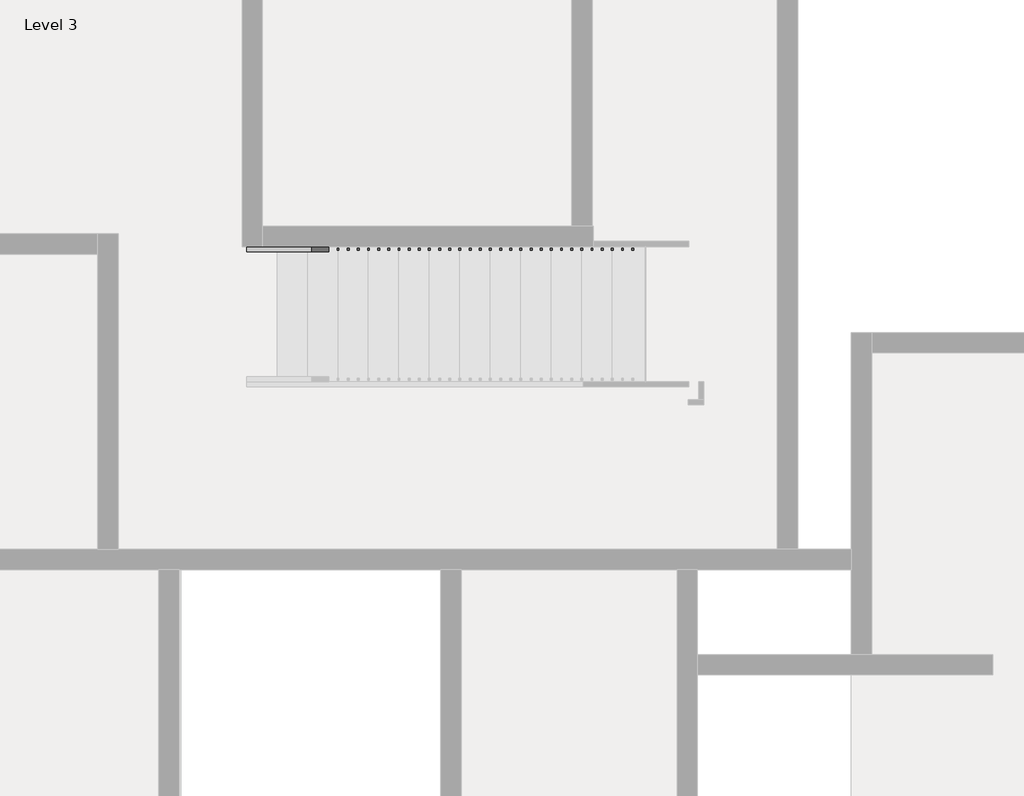
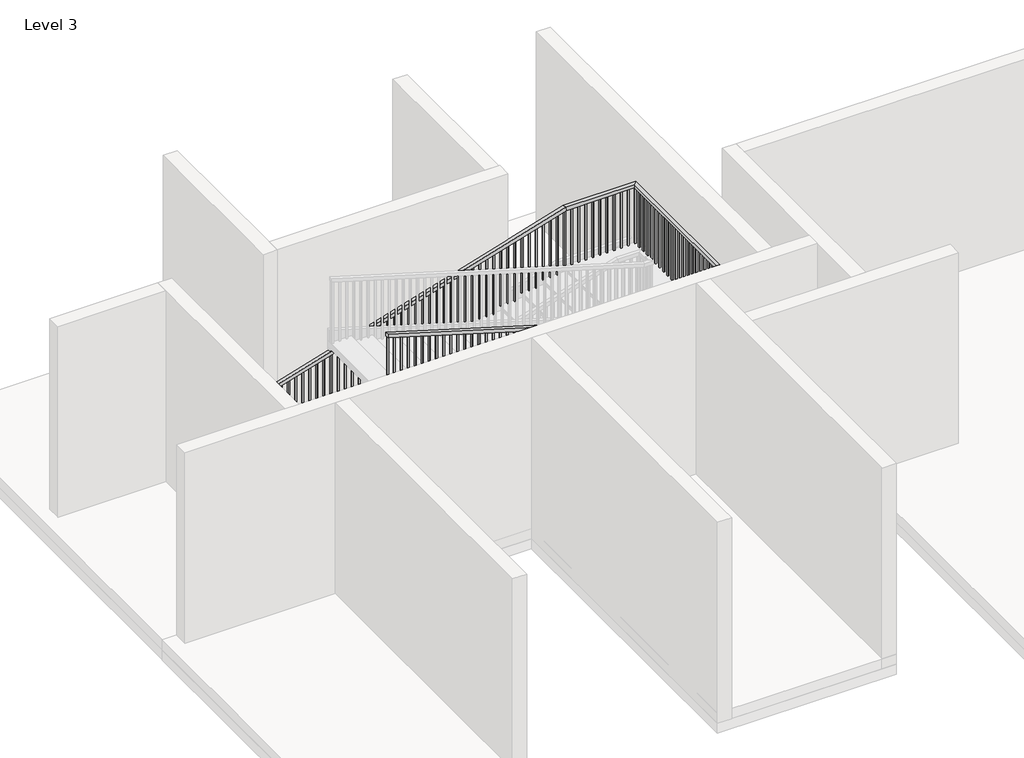
# One storey, part 10 of 14: 1 railing.
"""IFC4 building model written with IfcOpenShell, lengths in millimetres."""

from ifc_helpers import new_model, si_unit, frame, origin, place, context, project, spatial, polyline, outline, extrude, faceted_brep, element, save

model = new_model("IFC4")

# Units and contexts
model_context = context("Model", 3, world=origin())
ifc_project = project(units=[si_unit("LENGTHUNIT", "METRE", prefix="MILLI")], contexts=[model_context])

# Site, building, storey
site = spatial("IfcSite", under=ifc_project)
building = spatial("IfcBuilding", under=site)
storey = spatial("IfcBuildingStorey", under=building, Name="Level 3", Elevation=6096.0)

# Railing
placement = place(None, origin())
element("IfcRailing", 1, ObjectType="Handrail - Rectangular", at=placement, inside=storey, context=model_context, shape_type="SolidModel", body=[
    faceted_brep([(-5254.0891351, 12506.0715905, 7101.84), (-5254.0891351, 12506.0715905, 7048.8032429), (-5254.0891351, 12455.2715905, 7048.8032429), (-5254.0891351, 12455.2715905, 7101.84), (-986.8891351, 12506.0715905, 8382.0), (-979.4332782, 12506.0715905, 8331.2), (-979.4332782, 12455.2715905, 8331.2), (-986.8891351, 12455.2715905, 8382.0), (54.5108649, 12506.0715905, 8382.0), (54.5108649, 12506.0715905, 8331.2), (3.7108649, 12455.2715905, 8331.2), (3.7108649, 12455.2715905, 8382.0), (54.5108649, 9478.4949943, 8382.0), (54.5108649, 9478.4949943, 8331.2), (3.7108649, 9529.2949943, 8331.2), (3.7108649, 9529.2949943, 8382.0), (-682.0891351, 9478.4949943, 8382.0), (-689.544992, 9478.4949943, 8331.2), (-689.544992, 9529.2949943, 8331.2), (-682.0891351, 9529.2949943, 8382.0), (-5254.0891351, 9478.4949943, 9753.6), (-5254.0891351, 9529.2949943, 9753.6), (-5254.0891351, 9529.2949943, 9700.5632429), (-5254.0891351, 9478.4949943, 9700.5632429)], [[[0, 1, 2, 3]], [[1, 0, 4, 5]], [[2, 1, 5, 6]], [[3, 2, 6, 7]], [[0, 3, 7, 4]], [[5, 4, 8, 9]], [[6, 5, 9, 10]], [[7, 6, 10, 11]], [[4, 7, 11, 8]], [[9, 8, 12, 13]], [[10, 9, 13, 14]], [[11, 10, 14, 15]], [[8, 11, 15, 12]], [[13, 12, 16, 17]], [[14, 13, 17, 18]], [[15, 14, 18, 19]], [[12, 15, 19, 16]], [[20, 21, 22, 23]], [[17, 16, 20, 23]], [[18, 17, 23, 22]], [[19, 18, 22, 21]], [[16, 19, 21, 20]]]),
    extrude(outline(polyline([(9672.9407429, -5162.0141351), (8747.76, -5162.0141351), (8747.76, -5142.9641351), (9667.2257429, -5142.9641351), (9672.9407429, -5162.0141351)])), frame((0.0, 9494.3699943, 0.0), z_axis=(0.0, 1.0, 0.0), x_axis=(0.0, 0.0, 1.0)), (0.0, 0.0, 1.0), 19.05),
    extrude(outline(polyline([(9642.4607429, -5060.4141351), (8747.76, -5060.4141351), (8747.76, -5041.3641351), (9636.7457429, -5041.3641351), (9642.4607429, -5060.4141351)])), frame((0.0, 9494.3699943, 0.0), z_axis=(0.0, 1.0, 0.0), x_axis=(0.0, 0.0, 1.0)), (0.0, 0.0, 1.0), 19.05),
    extrude(outline(polyline([(9611.9807429, -4958.8141351), (8747.76, -4958.8141351), (8747.76, -4939.7641351), (9606.2657429, -4939.7641351), (9611.9807429, -4958.8141351)])), frame((0.0, 9494.3699943, 0.0), z_axis=(0.0, 1.0, 0.0), x_axis=(0.0, 0.0, 1.0)), (0.0, 0.0, 1.0), 19.05),
    extrude(outline(polyline([(9581.5007429, -4857.2141351), (8656.32, -4857.2141351), (8656.32, -4838.1641351), (9575.7857429, -4838.1641351), (9581.5007429, -4857.2141351)])), frame((0.0, 9494.3699943, 0.0), z_axis=(0.0, 1.0, 0.0), x_axis=(0.0, 0.0, 1.0)), (0.0, 0.0, 1.0), 19.05),
    extrude(outline(polyline([(9551.0207429, -4755.6141351), (8656.32, -4755.6141351), (8656.32, -4736.5641351), (9545.3057429, -4736.5641351), (9551.0207429, -4755.6141351)])), frame((0.0, 9494.3699943, 0.0), z_axis=(0.0, 1.0, 0.0), x_axis=(0.0, 0.0, 1.0)), (0.0, 0.0, 1.0), 19.05),
    extrude(outline(polyline([(9520.5407429, -4654.0141351), (8656.32, -4654.0141351), (8656.32, -4634.9641351), (9514.8257429, -4634.9641351), (9520.5407429, -4654.0141351)])), frame((0.0, 9494.3699943, 0.0), z_axis=(0.0, 1.0, 0.0), x_axis=(0.0, 0.0, 1.0)), (0.0, 0.0, 1.0), 19.05),
    extrude(outline(polyline([(9490.0607429, -4552.4141351), (8564.88, -4552.4141351), (8564.88, -4533.3641351), (9484.3457429, -4533.3641351), (9490.0607429, -4552.4141351)])), frame((0.0, 9494.3699943, 0.0), z_axis=(0.0, 1.0, 0.0), x_axis=(0.0, 0.0, 1.0)), (0.0, 0.0, 1.0), 19.05),
    extrude(outline(polyline([(9459.5807429, -4450.8141351), (8564.88, -4450.8141351), (8564.88, -4431.7641351), (9453.8657429, -4431.7641351), (9459.5807429, -4450.8141351)])), frame((0.0, 9494.3699943, 0.0), z_axis=(0.0, 1.0, 0.0), x_axis=(0.0, 0.0, 1.0)), (0.0, 0.0, 1.0), 19.05),
    extrude(outline(polyline([(9429.1007429, -4349.2141351), (8564.88, -4349.2141351), (8564.88, -4330.1641351), (9423.3857429, -4330.1641351), (9429.1007429, -4349.2141351)])), frame((0.0, 9494.3699943, 0.0), z_axis=(0.0, 1.0, 0.0), x_axis=(0.0, 0.0, 1.0)), (0.0, 0.0, 1.0), 19.05),
    extrude(outline(polyline([(9398.6207429, -4247.6141351), (8473.44, -4247.6141351), (8473.44, -4228.5641351), (9392.9057429, -4228.5641351), (9398.6207429, -4247.6141351)])), frame((0.0, 9494.3699943, 0.0), z_axis=(0.0, 1.0, 0.0), x_axis=(0.0, 0.0, 1.0)), (0.0, 0.0, 1.0), 19.05),
    extrude(outline(polyline([(9368.1407429, -4146.0141351), (8473.44, -4146.0141351), (8473.44, -4126.9641351), (9362.4257429, -4126.9641351), (9368.1407429, -4146.0141351)])), frame((0.0, 9494.3699943, 0.0), z_axis=(0.0, 1.0, 0.0), x_axis=(0.0, 0.0, 1.0)), (0.0, 0.0, 1.0), 19.05),
    extrude(outline(polyline([(9337.6607429, -4044.4141351), (8473.44, -4044.4141351), (8473.44, -4025.3641351), (9331.9457429, -4025.3641351), (9337.6607429, -4044.4141351)])), frame((0.0, 9494.3699943, 0.0), z_axis=(0.0, 1.0, 0.0), x_axis=(0.0, 0.0, 1.0)), (0.0, 0.0, 1.0), 19.05),
    extrude(outline(polyline([(9307.1807429, -3942.8141351), (8382.0, -3942.8141351), (8382.0, -3923.7641351), (9301.4657429, -3923.7641351), (9307.1807429, -3942.8141351)])), frame((0.0, 9494.3699943, 0.0), z_axis=(0.0, 1.0, 0.0), x_axis=(0.0, 0.0, 1.0)), (0.0, 0.0, 1.0), 19.05),
    extrude(outline(polyline([(9276.7007429, -3841.2141351), (8382.0, -3841.2141351), (8382.0, -3822.1641351), (9270.9857429, -3822.1641351), (9276.7007429, -3841.2141351)])), frame((0.0, 9494.3699943, 0.0), z_axis=(0.0, 1.0, 0.0), x_axis=(0.0, 0.0, 1.0)), (0.0, 0.0, 1.0), 19.05),
    extrude(outline(polyline([(9246.2207429, -3739.6141351), (8382.0, -3739.6141351), (8382.0, -3720.5641351), (9240.5057429, -3720.5641351), (9246.2207429, -3739.6141351)])), frame((0.0, 9494.3699943, 0.0), z_axis=(0.0, 1.0, 0.0), x_axis=(0.0, 0.0, 1.0)), (0.0, 0.0, 1.0), 19.05),
    extrude(outline(polyline([(9215.7407429, -3638.0141351), (8290.56, -3638.0141351), (8290.56, -3618.9641351), (9210.0257429, -3618.9641351), (9215.7407429, -3638.0141351)])), frame((0.0, 9494.3699943, 0.0), z_axis=(0.0, 1.0, 0.0), x_axis=(0.0, 0.0, 1.0)), (0.0, 0.0, 1.0), 19.05),
    extrude(outline(polyline([(9185.2607429, -3536.4141351), (8290.56, -3536.4141351), (8290.56, -3517.3641351), (9179.5457429, -3517.3641351), (9185.2607429, -3536.4141351)])), frame((0.0, 9494.3699943, 0.0), z_axis=(0.0, 1.0, 0.0), x_axis=(0.0, 0.0, 1.0)), (0.0, 0.0, 1.0), 19.05),
    extrude(outline(polyline([(9154.7807429, -3434.8141351), (8290.56, -3434.8141351), (8290.56, -3415.7641351), (9149.0657429, -3415.7641351), (9154.7807429, -3434.8141351)])), frame((0.0, 9494.3699943, 0.0), z_axis=(0.0, 1.0, 0.0), x_axis=(0.0, 0.0, 1.0)), (0.0, 0.0, 1.0), 19.05),
    extrude(outline(polyline([(9124.3007429, -3333.2141351), (8199.12, -3333.2141351), (8199.12, -3314.1641351), (9118.5857429, -3314.1641351), (9124.3007429, -3333.2141351)])), frame((0.0, 9494.3699943, 0.0), z_axis=(0.0, 1.0, 0.0), x_axis=(0.0, 0.0, 1.0)), (0.0, 0.0, 1.0), 19.05),
    extrude(outline(polyline([(9093.8207429, -3231.6141351), (8199.12, -3231.6141351), (8199.12, -3212.5641351), (9088.1057429, -3212.5641351), (9093.8207429, -3231.6141351)])), frame((0.0, 9494.3699943, 0.0), z_axis=(0.0, 1.0, 0.0), x_axis=(0.0, 0.0, 1.0)), (0.0, 0.0, 1.0), 19.05),
    extrude(outline(polyline([(9063.3407429, -3130.0141351), (8199.12, -3130.0141351), (8199.12, -3110.9641351), (9057.6257429, -3110.9641351), (9063.3407429, -3130.0141351)])), frame((0.0, 9494.3699943, 0.0), z_axis=(0.0, 1.0, 0.0), x_axis=(0.0, 0.0, 1.0)), (0.0, 0.0, 1.0), 19.05),
    extrude(outline(polyline([(9032.8607429, -3028.4141351), (8107.68, -3028.4141351), (8107.68, -3009.3641351), (9027.1457429, -3009.3641351), (9032.8607429, -3028.4141351)])), frame((0.0, 9494.3699943, 0.0), z_axis=(0.0, 1.0, 0.0), x_axis=(0.0, 0.0, 1.0)), (0.0, 0.0, 1.0), 19.05),
    extrude(outline(polyline([(9002.3807429, -2926.8141351), (8107.68, -2926.8141351), (8107.68, -2907.7641351), (8996.6657429, -2907.7641351), (9002.3807429, -2926.8141351)])), frame((0.0, 9494.3699943, 0.0), z_axis=(0.0, 1.0, 0.0), x_axis=(0.0, 0.0, 1.0)), (0.0, 0.0, 1.0), 19.05),
    extrude(outline(polyline([(8971.9007429, -2825.2141351), (8107.68, -2825.2141351), (8107.68, -2806.1641351), (8966.1857429, -2806.1641351), (8971.9007429, -2825.2141351)])), frame((0.0, 9494.3699943, 0.0), z_axis=(0.0, 1.0, 0.0), x_axis=(0.0, 0.0, 1.0)), (0.0, 0.0, 1.0), 19.05),
    extrude(outline(polyline([(8941.4207429, -2723.6141351), (8016.24, -2723.6141351), (8016.24, -2704.5641351), (8935.7057429, -2704.5641351), (8941.4207429, -2723.6141351)])), frame((0.0, 9494.3699943, 0.0), z_axis=(0.0, 1.0, 0.0), x_axis=(0.0, 0.0, 1.0)), (0.0, 0.0, 1.0), 19.05),
    extrude(outline(polyline([(8910.9407429, -2622.0141351), (8016.24, -2622.0141351), (8016.24, -2602.9641351), (8905.2257429, -2602.9641351), (8910.9407429, -2622.0141351)])), frame((0.0, 9494.3699943, 0.0), z_axis=(0.0, 1.0, 0.0), x_axis=(0.0, 0.0, 1.0)), (0.0, 0.0, 1.0), 19.05),
    extrude(outline(polyline([(8880.4607429, -2520.4141351), (8016.24, -2520.4141351), (8016.24, -2501.3641351), (8874.7457429, -2501.3641351), (8880.4607429, -2520.4141351)])), frame((0.0, 9494.3699943, 0.0), z_axis=(0.0, 1.0, 0.0), x_axis=(0.0, 0.0, 1.0)), (0.0, 0.0, 1.0), 19.05),
    extrude(outline(polyline([(8849.9807429, -2418.8141351), (7924.8, -2418.8141351), (7924.8, -2399.7641351), (8844.2657429, -2399.7641351), (8849.9807429, -2418.8141351)])), frame((0.0, 9494.3699943, 0.0), z_axis=(0.0, 1.0, 0.0), x_axis=(0.0, 0.0, 1.0)), (0.0, 0.0, 1.0), 19.05),
    extrude(outline(polyline([(8819.5007429, -2317.2141351), (7924.8, -2317.2141351), (7924.8, -2298.1641351), (8813.7857429, -2298.1641351), (8819.5007429, -2317.2141351)])), frame((0.0, 9494.3699943, 0.0), z_axis=(0.0, 1.0, 0.0), x_axis=(0.0, 0.0, 1.0)), (0.0, 0.0, 1.0), 19.05),
    extrude(outline(polyline([(8789.0207429, -2215.6141351), (7924.8, -2215.6141351), (7924.8, -2196.5641351), (8783.3057429, -2196.5641351), (8789.0207429, -2215.6141351)])), frame((0.0, 9494.3699943, 0.0), z_axis=(0.0, 1.0, 0.0), x_axis=(0.0, 0.0, 1.0)), (0.0, 0.0, 1.0), 19.05),
    extrude(outline(polyline([(8758.5407429, -2114.0141351), (7833.36, -2114.0141351), (7833.36, -2094.9641351), (8752.8257429, -2094.9641351), (8758.5407429, -2114.0141351)])), frame((0.0, 9494.3699943, 0.0), z_axis=(0.0, 1.0, 0.0), x_axis=(0.0, 0.0, 1.0)), (0.0, 0.0, 1.0), 19.05),
    extrude(outline(polyline([(8728.0607429, -2012.4141351), (7833.36, -2012.4141351), (7833.36, -1993.3641351), (8722.3457429, -1993.3641351), (8728.0607429, -2012.4141351)])), frame((0.0, 9494.3699943, 0.0), z_axis=(0.0, 1.0, 0.0), x_axis=(0.0, 0.0, 1.0)), (0.0, 0.0, 1.0), 19.05),
    extrude(outline(polyline([(8697.5807429, -1910.8141351), (7833.36, -1910.8141351), (7833.36, -1891.7641351), (8691.8657429, -1891.7641351), (8697.5807429, -1910.8141351)])), frame((0.0, 9494.3699943, 0.0), z_axis=(0.0, 1.0, 0.0), x_axis=(0.0, 0.0, 1.0)), (0.0, 0.0, 1.0), 19.05),
    extrude(outline(polyline([(8667.1007429, -1809.2141351), (7741.92, -1809.2141351), (7741.92, -1790.1641351), (8661.3857429, -1790.1641351), (8667.1007429, -1809.2141351)])), frame((0.0, 9494.3699943, 0.0), z_axis=(0.0, 1.0, 0.0), x_axis=(0.0, 0.0, 1.0)), (0.0, 0.0, 1.0), 19.05),
    extrude(outline(polyline([(8636.6207429, -1707.6141351), (7741.92, -1707.6141351), (7741.92, -1688.5641351), (8630.9057429, -1688.5641351), (8636.6207429, -1707.6141351)])), frame((0.0, 9494.3699943, 0.0), z_axis=(0.0, 1.0, 0.0), x_axis=(0.0, 0.0, 1.0)), (0.0, 0.0, 1.0), 19.05),
    extrude(outline(polyline([(8606.1407429, -1606.0141351), (7741.92, -1606.0141351), (7741.92, -1586.9641351), (8600.4257429, -1586.9641351), (8606.1407429, -1606.0141351)])), frame((0.0, 9494.3699943, 0.0), z_axis=(0.0, 1.0, 0.0), x_axis=(0.0, 0.0, 1.0)), (0.0, 0.0, 1.0), 19.05),
    extrude(outline(polyline([(8575.6607429, -1504.4141351), (7650.48, -1504.4141351), (7650.48, -1485.3641351), (8569.9457429, -1485.3641351), (8575.6607429, -1504.4141351)])), frame((0.0, 9494.3699943, 0.0), z_axis=(0.0, 1.0, 0.0), x_axis=(0.0, 0.0, 1.0)), (0.0, 0.0, 1.0), 19.05),
    extrude(outline(polyline([(8545.1807429, -1402.8141351), (7650.48, -1402.8141351), (7650.48, -1383.7641351), (8539.4657429, -1383.7641351), (8545.1807429, -1402.8141351)])), frame((0.0, 9494.3699943, 0.0), z_axis=(0.0, 1.0, 0.0), x_axis=(0.0, 0.0, 1.0)), (0.0, 0.0, 1.0), 19.05),
    extrude(outline(polyline([(8514.7007429, -1301.2141351), (7650.48, -1301.2141351), (7650.48, -1282.1641351), (8508.9857429, -1282.1641351), (8514.7007429, -1301.2141351)])), frame((0.0, 9494.3699943, 0.0), z_axis=(0.0, 1.0, 0.0), x_axis=(0.0, 0.0, 1.0)), (0.0, 0.0, 1.0), 19.05),
    extrude(outline(polyline([(8484.2207429, -1199.6141351), (7559.04, -1199.6141351), (7559.04, -1180.5641351), (8478.5057429, -1180.5641351), (8484.2207429, -1199.6141351)])), frame((0.0, 9494.3699943, 0.0), z_axis=(0.0, 1.0, 0.0), x_axis=(0.0, 0.0, 1.0)), (0.0, 0.0, 1.0), 19.05),
    extrude(outline(polyline([(8453.7407429, -1098.0141351), (7559.04, -1098.0141351), (7559.04, -1078.9641351), (8448.0257429, -1078.9641351), (8453.7407429, -1098.0141351)])), frame((0.0, 9494.3699943, 0.0), z_axis=(0.0, 1.0, 0.0), x_axis=(0.0, 0.0, 1.0)), (0.0, 0.0, 1.0), 19.05),
    extrude(outline(polyline([(8423.2607429, -996.4141351), (7559.04, -996.4141351), (7559.04, -977.3641351), (8417.5457429, -977.3641351), (8423.2607429, -996.4141351)])), frame((0.0, 9494.3699943, 0.0), z_axis=(0.0, 1.0, 0.0), x_axis=(0.0, 0.0, 1.0)), (0.0, 0.0, 1.0), 19.05),
    extrude(outline(polyline([(8392.7807429, -894.8141351), (7467.6, -894.8141351), (7467.6, -875.7641351), (8387.0657429, -875.7641351), (8392.7807429, -894.8141351)])), frame((0.0, 9494.3699943, 0.0), z_axis=(0.0, 1.0, 0.0), x_axis=(0.0, 0.0, 1.0)), (0.0, 0.0, 1.0), 19.05),
    extrude(outline(polyline([(8362.3007429, -793.2141351), (7467.6, -793.2141351), (7467.6, -774.1641351), (8356.5857429, -774.1641351), (8362.3007429, -793.2141351)])), frame((0.0, 9494.3699943, 0.0), z_axis=(0.0, 1.0, 0.0), x_axis=(0.0, 0.0, 1.0)), (0.0, 0.0, 1.0), 19.05),
    extrude(outline(polyline([(-672.5641351, 9494.3699943), (-691.6141351, 9494.3699943), (-691.6141351, 9513.4199943), (-672.5641351, 9513.4199943), (-672.5641351, 9494.3699943)])), frame((0.0, 0.0, 7467.6), z_axis=(0.0, 0.0, 1.0), x_axis=(1.0, 0.0, 0.0)), (0.0, 0.0, 1.0), 863.6),
    extrude(outline(polyline([(-570.9641351, 9494.3699943), (-590.0141351, 9494.3699943), (-590.0141351, 9513.4199943), (-570.9641351, 9513.4199943), (-570.9641351, 9494.3699943)])), frame((0.0, 0.0, 7467.6), z_axis=(0.0, 0.0, 1.0), x_axis=(1.0, 0.0, 0.0)), (0.0, 0.0, 1.0), 863.6),
    extrude(outline(polyline([(-469.3641351, 9494.3699943), (-488.4141351, 9494.3699943), (-488.4141351, 9513.4199943), (-469.3641351, 9513.4199943), (-469.3641351, 9494.3699943)])), frame((0.0, 0.0, 7467.6), z_axis=(0.0, 0.0, 1.0), x_axis=(1.0, 0.0, 0.0)), (0.0, 0.0, 1.0), 863.6),
    extrude(outline(polyline([(-367.7641351, 9494.3699943), (-386.8141351, 9494.3699943), (-386.8141351, 9513.4199943), (-367.7641351, 9513.4199943), (-367.7641351, 9494.3699943)])), frame((0.0, 0.0, 7467.6), z_axis=(0.0, 0.0, 1.0), x_axis=(1.0, 0.0, 0.0)), (0.0, 0.0, 1.0), 863.6),
    extrude(outline(polyline([(-266.1641351, 9494.3699943), (-285.2141351, 9494.3699943), (-285.2141351, 9513.4199943), (-266.1641351, 9513.4199943), (-266.1641351, 9494.3699943)])), frame((0.0, 0.0, 7467.6), z_axis=(0.0, 0.0, 1.0), x_axis=(1.0, 0.0, 0.0)), (0.0, 0.0, 1.0), 863.6),
    extrude(outline(polyline([(-164.5641351, 9494.3699943), (-183.6141351, 9494.3699943), (-183.6141351, 9513.4199943), (-164.5641351, 9513.4199943), (-164.5641351, 9494.3699943)])), frame((0.0, 0.0, 7467.6), z_axis=(0.0, 0.0, 1.0), x_axis=(1.0, 0.0, 0.0)), (0.0, 0.0, 1.0), 863.6),
    extrude(outline(polyline([(-62.9641351, 9494.3699943), (-82.0141351, 9494.3699943), (-82.0141351, 9513.4199943), (-62.9641351, 9513.4199943), (-62.9641351, 9494.3699943)])), frame((0.0, 0.0, 7467.6), z_axis=(0.0, 0.0, 1.0), x_axis=(1.0, 0.0, 0.0)), (0.0, 0.0, 1.0), 863.6),
    extrude(outline(polyline([(38.6358649, 9543.7965905), (38.6358649, 9524.7465905), (19.5858649, 9524.7465905), (19.5858649, 9543.7965905), (38.6358649, 9543.7965905)])), frame((0.0, 0.0, 7467.6), z_axis=(0.0, 0.0, 1.0), x_axis=(1.0, 0.0, 0.0)), (0.0, 0.0, 1.0), 863.6),
    extrude(outline(polyline([(38.6358649, 9645.3965905), (38.6358649, 9626.3465905), (19.5858649, 9626.3465905), (19.5858649, 9645.3965905), (38.6358649, 9645.3965905)])), frame((0.0, 0.0, 7467.6), z_axis=(0.0, 0.0, 1.0), x_axis=(1.0, 0.0, 0.0)), (0.0, 0.0, 1.0), 863.6),
    extrude(outline(polyline([(38.6358649, 9746.9965905), (38.6358649, 9727.9465905), (19.5858649, 9727.9465905), (19.5858649, 9746.9965905), (38.6358649, 9746.9965905)])), frame((0.0, 0.0, 7467.6), z_axis=(0.0, 0.0, 1.0), x_axis=(1.0, 0.0, 0.0)), (0.0, 0.0, 1.0), 863.6),
    extrude(outline(polyline([(38.6358649, 9848.5965905), (38.6358649, 9829.5465905), (19.5858649, 9829.5465905), (19.5858649, 9848.5965905), (38.6358649, 9848.5965905)])), frame((0.0, 0.0, 7467.6), z_axis=(0.0, 0.0, 1.0), x_axis=(1.0, 0.0, 0.0)), (0.0, 0.0, 1.0), 863.6),
    extrude(outline(polyline([(38.6358649, 9950.1965905), (38.6358649, 9931.1465905), (19.5858649, 9931.1465905), (19.5858649, 9950.1965905), (38.6358649, 9950.1965905)])), frame((0.0, 0.0, 7467.6), z_axis=(0.0, 0.0, 1.0), x_axis=(1.0, 0.0, 0.0)), (0.0, 0.0, 1.0), 863.6),
    extrude(outline(polyline([(38.6358649, 10051.7965905), (38.6358649, 10032.7465905), (19.5858649, 10032.7465905), (19.5858649, 10051.7965905), (38.6358649, 10051.7965905)])), frame((0.0, 0.0, 7467.6), z_axis=(0.0, 0.0, 1.0), x_axis=(1.0, 0.0, 0.0)), (0.0, 0.0, 1.0), 863.6),
    extrude(outline(polyline([(38.6358649, 10153.3965905), (38.6358649, 10134.3465905), (19.5858649, 10134.3465905), (19.5858649, 10153.3965905), (38.6358649, 10153.3965905)])), frame((0.0, 0.0, 7467.6), z_axis=(0.0, 0.0, 1.0), x_axis=(1.0, 0.0, 0.0)), (0.0, 0.0, 1.0), 863.6),
    extrude(outline(polyline([(38.6358649, 10254.9965905), (38.6358649, 10235.9465905), (19.5858649, 10235.9465905), (19.5858649, 10254.9965905), (38.6358649, 10254.9965905)])), frame((0.0, 0.0, 7467.6), z_axis=(0.0, 0.0, 1.0), x_axis=(1.0, 0.0, 0.0)), (0.0, 0.0, 1.0), 863.6),
    extrude(outline(polyline([(38.6358649, 10356.5965905), (38.6358649, 10337.5465905), (19.5858649, 10337.5465905), (19.5858649, 10356.5965905), (38.6358649, 10356.5965905)])), frame((0.0, 0.0, 7467.6), z_axis=(0.0, 0.0, 1.0), x_axis=(1.0, 0.0, 0.0)), (0.0, 0.0, 1.0), 863.6),
    extrude(outline(polyline([(38.6358649, 10458.1965905), (38.6358649, 10439.1465905), (19.5858649, 10439.1465905), (19.5858649, 10458.1965905), (38.6358649, 10458.1965905)])), frame((0.0, 0.0, 7467.6), z_axis=(0.0, 0.0, 1.0), x_axis=(1.0, 0.0, 0.0)), (0.0, 0.0, 1.0), 863.6),
    extrude(outline(polyline([(38.6358649, 10559.7965905), (38.6358649, 10540.7465905), (19.5858649, 10540.7465905), (19.5858649, 10559.7965905), (38.6358649, 10559.7965905)])), frame((0.0, 0.0, 7467.6), z_axis=(0.0, 0.0, 1.0), x_axis=(1.0, 0.0, 0.0)), (0.0, 0.0, 1.0), 863.6),
    extrude(outline(polyline([(38.6358649, 10661.3965905), (38.6358649, 10642.3465905), (19.5858649, 10642.3465905), (19.5858649, 10661.3965905), (38.6358649, 10661.3965905)])), frame((0.0, 0.0, 7467.6), z_axis=(0.0, 0.0, 1.0), x_axis=(1.0, 0.0, 0.0)), (0.0, 0.0, 1.0), 863.6),
    extrude(outline(polyline([(38.6358649, 10762.9965905), (38.6358649, 10743.9465905), (19.5858649, 10743.9465905), (19.5858649, 10762.9965905), (38.6358649, 10762.9965905)])), frame((0.0, 0.0, 7467.6), z_axis=(0.0, 0.0, 1.0), x_axis=(1.0, 0.0, 0.0)), (0.0, 0.0, 1.0), 863.6),
    extrude(outline(polyline([(38.6358649, 10864.5965905), (38.6358649, 10845.5465905), (19.5858649, 10845.5465905), (19.5858649, 10864.5965905), (38.6358649, 10864.5965905)])), frame((0.0, 0.0, 7467.6), z_axis=(0.0, 0.0, 1.0), x_axis=(1.0, 0.0, 0.0)), (0.0, 0.0, 1.0), 863.6),
    extrude(outline(polyline([(38.6358649, 10966.1965905), (38.6358649, 10947.1465905), (19.5858649, 10947.1465905), (19.5858649, 10966.1965905), (38.6358649, 10966.1965905)])), frame((0.0, 0.0, 7467.6), z_axis=(0.0, 0.0, 1.0), x_axis=(1.0, 0.0, 0.0)), (0.0, 0.0, 1.0), 863.6),
    extrude(outline(polyline([(38.6358649, 11067.7965905), (38.6358649, 11048.7465905), (19.5858649, 11048.7465905), (19.5858649, 11067.7965905), (38.6358649, 11067.7965905)])), frame((0.0, 0.0, 7467.6), z_axis=(0.0, 0.0, 1.0), x_axis=(1.0, 0.0, 0.0)), (0.0, 0.0, 1.0), 863.6),
    extrude(outline(polyline([(38.6358649, 11169.3965905), (38.6358649, 11150.3465905), (19.5858649, 11150.3465905), (19.5858649, 11169.3965905), (38.6358649, 11169.3965905)])), frame((0.0, 0.0, 7467.6), z_axis=(0.0, 0.0, 1.0), x_axis=(1.0, 0.0, 0.0)), (0.0, 0.0, 1.0), 863.6),
    extrude(outline(polyline([(38.6358649, 11270.9965905), (38.6358649, 11251.9465905), (19.5858649, 11251.9465905), (19.5858649, 11270.9965905), (38.6358649, 11270.9965905)])), frame((0.0, 0.0, 7467.6), z_axis=(0.0, 0.0, 1.0), x_axis=(1.0, 0.0, 0.0)), (0.0, 0.0, 1.0), 863.6),
    extrude(outline(polyline([(38.6358649, 11372.5965905), (38.6358649, 11353.5465905), (19.5858649, 11353.5465905), (19.5858649, 11372.5965905), (38.6358649, 11372.5965905)])), frame((0.0, 0.0, 7467.6), z_axis=(0.0, 0.0, 1.0), x_axis=(1.0, 0.0, 0.0)), (0.0, 0.0, 1.0), 863.6),
    extrude(outline(polyline([(38.6358649, 11474.1965905), (38.6358649, 11455.1465905), (19.5858649, 11455.1465905), (19.5858649, 11474.1965905), (38.6358649, 11474.1965905)])), frame((0.0, 0.0, 7467.6), z_axis=(0.0, 0.0, 1.0), x_axis=(1.0, 0.0, 0.0)), (0.0, 0.0, 1.0), 863.6),
    extrude(outline(polyline([(38.6358649, 11575.7965905), (38.6358649, 11556.7465905), (19.5858649, 11556.7465905), (19.5858649, 11575.7965905), (38.6358649, 11575.7965905)])), frame((0.0, 0.0, 7467.6), z_axis=(0.0, 0.0, 1.0), x_axis=(1.0, 0.0, 0.0)), (0.0, 0.0, 1.0), 863.6),
    extrude(outline(polyline([(38.6358649, 11677.3965905), (38.6358649, 11658.3465905), (19.5858649, 11658.3465905), (19.5858649, 11677.3965905), (38.6358649, 11677.3965905)])), frame((0.0, 0.0, 7467.6), z_axis=(0.0, 0.0, 1.0), x_axis=(1.0, 0.0, 0.0)), (0.0, 0.0, 1.0), 863.6),
    extrude(outline(polyline([(38.6358649, 11778.9965905), (38.6358649, 11759.9465905), (19.5858649, 11759.9465905), (19.5858649, 11778.9965905), (38.6358649, 11778.9965905)])), frame((0.0, 0.0, 7467.6), z_axis=(0.0, 0.0, 1.0), x_axis=(1.0, 0.0, 0.0)), (0.0, 0.0, 1.0), 863.6),
    extrude(outline(polyline([(38.6358649, 11880.5965905), (38.6358649, 11861.5465905), (19.5858649, 11861.5465905), (19.5858649, 11880.5965905), (38.6358649, 11880.5965905)])), frame((0.0, 0.0, 7467.6), z_axis=(0.0, 0.0, 1.0), x_axis=(1.0, 0.0, 0.0)), (0.0, 0.0, 1.0), 863.6),
    extrude(outline(polyline([(38.6358649, 11982.1965905), (38.6358649, 11963.1465905), (19.5858649, 11963.1465905), (19.5858649, 11982.1965905), (38.6358649, 11982.1965905)])), frame((0.0, 0.0, 7467.6), z_axis=(0.0, 0.0, 1.0), x_axis=(1.0, 0.0, 0.0)), (0.0, 0.0, 1.0), 863.6),
    extrude(outline(polyline([(38.6358649, 12083.7965905), (38.6358649, 12064.7465905), (19.5858649, 12064.7465905), (19.5858649, 12083.7965905), (38.6358649, 12083.7965905)])), frame((0.0, 0.0, 7467.6), z_axis=(0.0, 0.0, 1.0), x_axis=(1.0, 0.0, 0.0)), (0.0, 0.0, 1.0), 863.6),
    extrude(outline(polyline([(38.6358649, 12185.3965905), (38.6358649, 12166.3465905), (19.5858649, 12166.3465905), (19.5858649, 12185.3965905), (38.6358649, 12185.3965905)])), frame((0.0, 0.0, 7467.6), z_axis=(0.0, 0.0, 1.0), x_axis=(1.0, 0.0, 0.0)), (0.0, 0.0, 1.0), 863.6),
    extrude(outline(polyline([(38.6358649, 12286.9965905), (38.6358649, 12267.9465905), (19.5858649, 12267.9465905), (19.5858649, 12286.9965905), (38.6358649, 12286.9965905)])), frame((0.0, 0.0, 7467.6), z_axis=(0.0, 0.0, 1.0), x_axis=(1.0, 0.0, 0.0)), (0.0, 0.0, 1.0), 863.6),
    extrude(outline(polyline([(38.6358649, 12388.5965905), (38.6358649, 12369.5465905), (19.5858649, 12369.5465905), (19.5858649, 12388.5965905), (38.6358649, 12388.5965905)])), frame((0.0, 0.0, 7467.6), z_axis=(0.0, 0.0, 1.0), x_axis=(1.0, 0.0, 0.0)), (0.0, 0.0, 1.0), 863.6),
    extrude(outline(polyline([(-82.0141351, 12490.1965905), (-62.9641351, 12490.1965905), (-62.9641351, 12471.1465905), (-82.0141351, 12471.1465905), (-82.0141351, 12490.1965905)])), frame((0.0, 0.0, 7467.6), z_axis=(0.0, 0.0, 1.0), x_axis=(1.0, 0.0, 0.0)), (0.0, 0.0, 1.0), 863.6),
    extrude(outline(polyline([(-183.6141351, 12490.1965905), (-164.5641351, 12490.1965905), (-164.5641351, 12471.1465905), (-183.6141351, 12471.1465905), (-183.6141351, 12490.1965905)])), frame((0.0, 0.0, 7467.6), z_axis=(0.0, 0.0, 1.0), x_axis=(1.0, 0.0, 0.0)), (0.0, 0.0, 1.0), 863.6),
    extrude(outline(polyline([(-285.2141351, 12490.1965905), (-266.1641351, 12490.1965905), (-266.1641351, 12471.1465905), (-285.2141351, 12471.1465905), (-285.2141351, 12490.1965905)])), frame((0.0, 0.0, 7467.6), z_axis=(0.0, 0.0, 1.0), x_axis=(1.0, 0.0, 0.0)), (0.0, 0.0, 1.0), 863.6),
    extrude(outline(polyline([(-386.8141351, 12490.1965905), (-367.7641351, 12490.1965905), (-367.7641351, 12471.1465905), (-386.8141351, 12471.1465905), (-386.8141351, 12490.1965905)])), frame((0.0, 0.0, 7467.6), z_axis=(0.0, 0.0, 1.0), x_axis=(1.0, 0.0, 0.0)), (0.0, 0.0, 1.0), 863.6),
    extrude(outline(polyline([(-488.4141351, 12490.1965905), (-469.3641351, 12490.1965905), (-469.3641351, 12471.1465905), (-488.4141351, 12471.1465905), (-488.4141351, 12490.1965905)])), frame((0.0, 0.0, 7467.6), z_axis=(0.0, 0.0, 1.0), x_axis=(1.0, 0.0, 0.0)), (0.0, 0.0, 1.0), 863.6),
    extrude(outline(polyline([(-590.0141351, 12490.1965905), (-570.9641351, 12490.1965905), (-570.9641351, 12471.1465905), (-590.0141351, 12471.1465905), (-590.0141351, 12490.1965905)])), frame((0.0, 0.0, 7467.6), z_axis=(0.0, 0.0, 1.0), x_axis=(1.0, 0.0, 0.0)), (0.0, 0.0, 1.0), 863.6),
    extrude(outline(polyline([(-691.6141351, 12490.1965905), (-672.5641351, 12490.1965905), (-672.5641351, 12471.1465905), (-691.6141351, 12471.1465905), (-691.6141351, 12490.1965905)])), frame((0.0, 0.0, 7467.6), z_axis=(0.0, 0.0, 1.0), x_axis=(1.0, 0.0, 0.0)), (0.0, 0.0, 1.0), 863.6),
    extrude(outline(polyline([(-793.2141351, 12490.1965905), (-774.1641351, 12490.1965905), (-774.1641351, 12471.1465905), (-793.2141351, 12471.1465905), (-793.2141351, 12490.1965905)])), frame((0.0, 0.0, 7467.6), z_axis=(0.0, 0.0, 1.0), x_axis=(1.0, 0.0, 0.0)), (0.0, 0.0, 1.0), 863.6),
    extrude(outline(polyline([(-894.8141351, 12490.1965905), (-875.7641351, 12490.1965905), (-875.7641351, 12471.1465905), (-894.8141351, 12471.1465905), (-894.8141351, 12490.1965905)])), frame((0.0, 0.0, 7467.6), z_axis=(0.0, 0.0, 1.0), x_axis=(1.0, 0.0, 0.0)), (0.0, 0.0, 1.0), 863.6),
    extrude(outline(polyline([(8326.1057429, -996.4141351), (7467.6, -996.4141351), (7467.6, -977.3641351), (8331.8207429, -977.3641351), (8326.1057429, -996.4141351)])), frame((0.0, 12471.1465905, 0.0), z_axis=(0.0, 1.0, 0.0), x_axis=(0.0, 0.0, 1.0)), (0.0, 0.0, 1.0), 19.05),
    extrude(outline(polyline([(8295.6257429, -1098.0141351), (7376.16, -1098.0141351), (7376.16, -1078.9641351), (8301.3407429, -1078.9641351), (8295.6257429, -1098.0141351)])), frame((0.0, 12471.1465905, 0.0), z_axis=(0.0, 1.0, 0.0), x_axis=(0.0, 0.0, 1.0)), (0.0, 0.0, 1.0), 19.05),
    extrude(outline(polyline([(8265.1457429, -1199.6141351), (7376.16, -1199.6141351), (7376.16, -1180.5641351), (8270.8607429, -1180.5641351), (8265.1457429, -1199.6141351)])), frame((0.0, 12471.1465905, 0.0), z_axis=(0.0, 1.0, 0.0), x_axis=(0.0, 0.0, 1.0)), (0.0, 0.0, 1.0), 19.05),
    extrude(outline(polyline([(8234.6657429, -1301.2141351), (7376.16, -1301.2141351), (7376.16, -1282.1641351), (8240.3807429, -1282.1641351), (8234.6657429, -1301.2141351)])), frame((0.0, 12471.1465905, 0.0), z_axis=(0.0, 1.0, 0.0), x_axis=(0.0, 0.0, 1.0)), (0.0, 0.0, 1.0), 19.05),
    extrude(outline(polyline([(8204.1857429, -1402.8141351), (7284.72, -1402.8141351), (7284.72, -1383.7641351), (8209.9007429, -1383.7641351), (8204.1857429, -1402.8141351)])), frame((0.0, 12471.1465905, 0.0), z_axis=(0.0, 1.0, 0.0), x_axis=(0.0, 0.0, 1.0)), (0.0, 0.0, 1.0), 19.05),
    extrude(outline(polyline([(8173.7057429, -1504.4141351), (7284.72, -1504.4141351), (7284.72, -1485.3641351), (8179.4207429, -1485.3641351), (8173.7057429, -1504.4141351)])), frame((0.0, 12471.1465905, 0.0), z_axis=(0.0, 1.0, 0.0), x_axis=(0.0, 0.0, 1.0)), (0.0, 0.0, 1.0), 19.05),
    extrude(outline(polyline([(8143.2257429, -1606.0141351), (7284.72, -1606.0141351), (7284.72, -1586.9641351), (8148.9407429, -1586.9641351), (8143.2257429, -1606.0141351)])), frame((0.0, 12471.1465905, 0.0), z_axis=(0.0, 1.0, 0.0), x_axis=(0.0, 0.0, 1.0)), (0.0, 0.0, 1.0), 19.05),
    extrude(outline(polyline([(8112.7457429, -1707.6141351), (7193.28, -1707.6141351), (7193.28, -1688.5641351), (8118.4607429, -1688.5641351), (8112.7457429, -1707.6141351)])), frame((0.0, 12471.1465905, 0.0), z_axis=(0.0, 1.0, 0.0), x_axis=(0.0, 0.0, 1.0)), (0.0, 0.0, 1.0), 19.05),
    extrude(outline(polyline([(8082.2657429, -1809.2141351), (7193.28, -1809.2141351), (7193.28, -1790.1641351), (8087.9807429, -1790.1641351), (8082.2657429, -1809.2141351)])), frame((0.0, 12471.1465905, 0.0), z_axis=(0.0, 1.0, 0.0), x_axis=(0.0, 0.0, 1.0)), (0.0, 0.0, 1.0), 19.05),
    extrude(outline(polyline([(8051.7857429, -1910.8141351), (7193.28, -1910.8141351), (7193.28, -1891.7641351), (8057.5007429, -1891.7641351), (8051.7857429, -1910.8141351)])), frame((0.0, 12471.1465905, 0.0), z_axis=(0.0, 1.0, 0.0), x_axis=(0.0, 0.0, 1.0)), (0.0, 0.0, 1.0), 19.05),
    extrude(outline(polyline([(8021.3057429, -2012.4141351), (7101.84, -2012.4141351), (7101.84, -1993.3641351), (8027.0207429, -1993.3641351), (8021.3057429, -2012.4141351)])), frame((0.0, 12471.1465905, 0.0), z_axis=(0.0, 1.0, 0.0), x_axis=(0.0, 0.0, 1.0)), (0.0, 0.0, 1.0), 19.05),
    extrude(outline(polyline([(7990.8257429, -2114.0141351), (7101.84, -2114.0141351), (7101.84, -2094.9641351), (7996.5407429, -2094.9641351), (7990.8257429, -2114.0141351)])), frame((0.0, 12471.1465905, 0.0), z_axis=(0.0, 1.0, 0.0), x_axis=(0.0, 0.0, 1.0)), (0.0, 0.0, 1.0), 19.05),
    extrude(outline(polyline([(7960.3457429, -2215.6141351), (7101.84, -2215.6141351), (7101.84, -2196.5641351), (7966.0607429, -2196.5641351), (7960.3457429, -2215.6141351)])), frame((0.0, 12471.1465905, 0.0), z_axis=(0.0, 1.0, 0.0), x_axis=(0.0, 0.0, 1.0)), (0.0, 0.0, 1.0), 19.05),
    extrude(outline(polyline([(7929.8657429, -2317.2141351), (7010.4, -2317.2141351), (7010.4, -2298.1641351), (7935.5807429, -2298.1641351), (7929.8657429, -2317.2141351)])), frame((0.0, 12471.1465905, 0.0), z_axis=(0.0, 1.0, 0.0), x_axis=(0.0, 0.0, 1.0)), (0.0, 0.0, 1.0), 19.05),
    extrude(outline(polyline([(7899.3857429, -2418.8141351), (7010.4, -2418.8141351), (7010.4, -2399.7641351), (7905.1007429, -2399.7641351), (7899.3857429, -2418.8141351)])), frame((0.0, 12471.1465905, 0.0), z_axis=(0.0, 1.0, 0.0), x_axis=(0.0, 0.0, 1.0)), (0.0, 0.0, 1.0), 19.05),
    extrude(outline(polyline([(7868.9057429, -2520.4141351), (7010.4, -2520.4141351), (7010.4, -2501.3641351), (7874.6207429, -2501.3641351), (7868.9057429, -2520.4141351)])), frame((0.0, 12471.1465905, 0.0), z_axis=(0.0, 1.0, 0.0), x_axis=(0.0, 0.0, 1.0)), (0.0, 0.0, 1.0), 19.05),
    extrude(outline(polyline([(7838.4257429, -2622.0141351), (6918.96, -2622.0141351), (6918.96, -2602.9641351), (7844.1407429, -2602.9641351), (7838.4257429, -2622.0141351)])), frame((0.0, 12471.1465905, 0.0), z_axis=(0.0, 1.0, 0.0), x_axis=(0.0, 0.0, 1.0)), (0.0, 0.0, 1.0), 19.05),
    extrude(outline(polyline([(7807.9457429, -2723.6141351), (6918.96, -2723.6141351), (6918.96, -2704.5641351), (7813.6607429, -2704.5641351), (7807.9457429, -2723.6141351)])), frame((0.0, 12471.1465905, 0.0), z_axis=(0.0, 1.0, 0.0), x_axis=(0.0, 0.0, 1.0)), (0.0, 0.0, 1.0), 19.05),
    extrude(outline(polyline([(7777.4657429, -2825.2141351), (6918.96, -2825.2141351), (6918.96, -2806.1641351), (7783.1807429, -2806.1641351), (7777.4657429, -2825.2141351)])), frame((0.0, 12471.1465905, 0.0), z_axis=(0.0, 1.0, 0.0), x_axis=(0.0, 0.0, 1.0)), (0.0, 0.0, 1.0), 19.05),
    extrude(outline(polyline([(7746.9857429, -2926.8141351), (6827.52, -2926.8141351), (6827.52, -2907.7641351), (7752.7007429, -2907.7641351), (7746.9857429, -2926.8141351)])), frame((0.0, 12471.1465905, 0.0), z_axis=(0.0, 1.0, 0.0), x_axis=(0.0, 0.0, 1.0)), (0.0, 0.0, 1.0), 19.05),
    extrude(outline(polyline([(7716.5057429, -3028.4141351), (6827.52, -3028.4141351), (6827.52, -3009.3641351), (7722.2207429, -3009.3641351), (7716.5057429, -3028.4141351)])), frame((0.0, 12471.1465905, 0.0), z_axis=(0.0, 1.0, 0.0), x_axis=(0.0, 0.0, 1.0)), (0.0, 0.0, 1.0), 19.05),
    extrude(outline(polyline([(7686.0257429, -3130.0141351), (6827.52, -3130.0141351), (6827.52, -3110.9641351), (7691.7407429, -3110.9641351), (7686.0257429, -3130.0141351)])), frame((0.0, 12471.1465905, 0.0), z_axis=(0.0, 1.0, 0.0), x_axis=(0.0, 0.0, 1.0)), (0.0, 0.0, 1.0), 19.05),
    extrude(outline(polyline([(7655.5457429, -3231.6141351), (6736.08, -3231.6141351), (6736.08, -3212.5641351), (7661.2607429, -3212.5641351), (7655.5457429, -3231.6141351)])), frame((0.0, 12471.1465905, 0.0), z_axis=(0.0, 1.0, 0.0), x_axis=(0.0, 0.0, 1.0)), (0.0, 0.0, 1.0), 19.05),
    extrude(outline(polyline([(7625.0657429, -3333.2141351), (6736.08, -3333.2141351), (6736.08, -3314.1641351), (7630.7807429, -3314.1641351), (7625.0657429, -3333.2141351)])), frame((0.0, 12471.1465905, 0.0), z_axis=(0.0, 1.0, 0.0), x_axis=(0.0, 0.0, 1.0)), (0.0, 0.0, 1.0), 19.05),
    extrude(outline(polyline([(7594.5857429, -3434.8141351), (6736.08, -3434.8141351), (6736.08, -3415.7641351), (7600.3007429, -3415.7641351), (7594.5857429, -3434.8141351)])), frame((0.0, 12471.1465905, 0.0), z_axis=(0.0, 1.0, 0.0), x_axis=(0.0, 0.0, 1.0)), (0.0, 0.0, 1.0), 19.05),
    extrude(outline(polyline([(7564.1057429, -3536.4141351), (6644.64, -3536.4141351), (6644.64, -3517.3641351), (7569.8207429, -3517.3641351), (7564.1057429, -3536.4141351)])), frame((0.0, 12471.1465905, 0.0), z_axis=(0.0, 1.0, 0.0), x_axis=(0.0, 0.0, 1.0)), (0.0, 0.0, 1.0), 19.05),
    extrude(outline(polyline([(7533.6257429, -3638.0141351), (6644.64, -3638.0141351), (6644.64, -3618.9641351), (7539.3407429, -3618.9641351), (7533.6257429, -3638.0141351)])), frame((0.0, 12471.1465905, 0.0), z_axis=(0.0, 1.0, 0.0), x_axis=(0.0, 0.0, 1.0)), (0.0, 0.0, 1.0), 19.05),
    extrude(outline(polyline([(7503.1457429, -3739.6141351), (6644.64, -3739.6141351), (6644.64, -3720.5641351), (7508.8607429, -3720.5641351), (7503.1457429, -3739.6141351)])), frame((0.0, 12471.1465905, 0.0), z_axis=(0.0, 1.0, 0.0), x_axis=(0.0, 0.0, 1.0)), (0.0, 0.0, 1.0), 19.05),
    extrude(outline(polyline([(7472.6657429, -3841.2141351), (6553.2, -3841.2141351), (6553.2, -3822.1641351), (7478.3807429, -3822.1641351), (7472.6657429, -3841.2141351)])), frame((0.0, 12471.1465905, 0.0), z_axis=(0.0, 1.0, 0.0), x_axis=(0.0, 0.0, 1.0)), (0.0, 0.0, 1.0), 19.05),
    extrude(outline(polyline([(7442.1857429, -3942.8141351), (6553.2, -3942.8141351), (6553.2, -3923.7641351), (7447.9007429, -3923.7641351), (7442.1857429, -3942.8141351)])), frame((0.0, 12471.1465905, 0.0), z_axis=(0.0, 1.0, 0.0), x_axis=(0.0, 0.0, 1.0)), (0.0, 0.0, 1.0), 19.05),
    extrude(outline(polyline([(7411.7057429, -4044.4141351), (6553.2, -4044.4141351), (6553.2, -4025.3641351), (7417.4207429, -4025.3641351), (7411.7057429, -4044.4141351)])), frame((0.0, 12471.1465905, 0.0), z_axis=(0.0, 1.0, 0.0), x_axis=(0.0, 0.0, 1.0)), (0.0, 0.0, 1.0), 19.05),
    extrude(outline(polyline([(7381.2257429, -4146.0141351), (6461.76, -4146.0141351), (6461.76, -4126.9641351), (7386.9407429, -4126.9641351), (7381.2257429, -4146.0141351)])), frame((0.0, 12471.1465905, 0.0), z_axis=(0.0, 1.0, 0.0), x_axis=(0.0, 0.0, 1.0)), (0.0, 0.0, 1.0), 19.05),
    extrude(outline(polyline([(7350.7457429, -4247.6141351), (6461.76, -4247.6141351), (6461.76, -4228.5641351), (7356.4607429, -4228.5641351), (7350.7457429, -4247.6141351)])), frame((0.0, 12471.1465905, 0.0), z_axis=(0.0, 1.0, 0.0), x_axis=(0.0, 0.0, 1.0)), (0.0, 0.0, 1.0), 19.05),
    extrude(outline(polyline([(7320.2657429, -4349.2141351), (6461.76, -4349.2141351), (6461.76, -4330.1641351), (7325.9807429, -4330.1641351), (7320.2657429, -4349.2141351)])), frame((0.0, 12471.1465905, 0.0), z_axis=(0.0, 1.0, 0.0), x_axis=(0.0, 0.0, 1.0)), (0.0, 0.0, 1.0), 19.05),
    extrude(outline(polyline([(7289.7857429, -4450.8141351), (6370.32, -4450.8141351), (6370.32, -4431.7641351), (7295.5007429, -4431.7641351), (7289.7857429, -4450.8141351)])), frame((0.0, 12471.1465905, 0.0), z_axis=(0.0, 1.0, 0.0), x_axis=(0.0, 0.0, 1.0)), (0.0, 0.0, 1.0), 19.05),
    extrude(outline(polyline([(7259.3057429, -4552.4141351), (6370.32, -4552.4141351), (6370.32, -4533.3641351), (7265.0207429, -4533.3641351), (7259.3057429, -4552.4141351)])), frame((0.0, 12471.1465905, 0.0), z_axis=(0.0, 1.0, 0.0), x_axis=(0.0, 0.0, 1.0)), (0.0, 0.0, 1.0), 19.05),
    extrude(outline(polyline([(7228.8257429, -4654.0141351), (6370.32, -4654.0141351), (6370.32, -4634.9641351), (7234.5407429, -4634.9641351), (7228.8257429, -4654.0141351)])), frame((0.0, 12471.1465905, 0.0), z_axis=(0.0, 1.0, 0.0), x_axis=(0.0, 0.0, 1.0)), (0.0, 0.0, 1.0), 19.05),
    extrude(outline(polyline([(7198.3457429, -4755.6141351), (6278.88, -4755.6141351), (6278.88, -4736.5641351), (7204.0607429, -4736.5641351), (7198.3457429, -4755.6141351)])), frame((0.0, 12471.1465905, 0.0), z_axis=(0.0, 1.0, 0.0), x_axis=(0.0, 0.0, 1.0)), (0.0, 0.0, 1.0), 19.05),
    extrude(outline(polyline([(7167.8657429, -4857.2141351), (6278.88, -4857.2141351), (6278.88, -4838.1641351), (7173.5807429, -4838.1641351), (7167.8657429, -4857.2141351)])), frame((0.0, 12471.1465905, 0.0), z_axis=(0.0, 1.0, 0.0), x_axis=(0.0, 0.0, 1.0)), (0.0, 0.0, 1.0), 19.05),
    extrude(outline(polyline([(7137.3857429, -4958.8141351), (6278.88, -4958.8141351), (6278.88, -4939.7641351), (7143.1007429, -4939.7641351), (7137.3857429, -4958.8141351)])), frame((0.0, 12471.1465905, 0.0), z_axis=(0.0, 1.0, 0.0), x_axis=(0.0, 0.0, 1.0)), (0.0, 0.0, 1.0), 19.05),
    extrude(outline(polyline([(7106.9057429, -5060.4141351), (6187.44, -5060.4141351), (6187.44, -5041.3641351), (7112.6207429, -5041.3641351), (7106.9057429, -5060.4141351)])), frame((0.0, 12471.1465905, 0.0), z_axis=(0.0, 1.0, 0.0), x_axis=(0.0, 0.0, 1.0)), (0.0, 0.0, 1.0), 19.05),
    extrude(outline(polyline([(7076.4257429, -5162.0141351), (6187.44, -5162.0141351), (6187.44, -5142.9641351), (7082.1407429, -5142.9641351), (7076.4257429, -5162.0141351)])), frame((0.0, 12471.1465905, 0.0), z_axis=(0.0, 1.0, 0.0), x_axis=(0.0, 0.0, 1.0)), (0.0, 0.0, 1.0), 19.05),
    extrude(outline(polyline([(38.6358649, 9513.4199943), (38.6358649, 9494.3699943), (19.5858649, 9494.3699943), (19.5858649, 9513.4199943), (38.6358649, 9513.4199943)])), frame((0.0, 0.0, 7467.6), z_axis=(0.0, 0.0, 1.0), x_axis=(1.0, 0.0, 0.0)), (0.0, 0.0, 1.0), 863.6),
    extrude(outline(polyline([(19.5858649, 12490.1965905), (38.6358649, 12490.1965905), (38.6358649, 12471.1465905), (19.5858649, 12471.1465905), (19.5858649, 12490.1965905)])), frame((0.0, 0.0, 7467.6), z_axis=(0.0, 0.0, 1.0), x_axis=(1.0, 0.0, 0.0)), (0.0, 0.0, 1.0), 863.6),
    extrude(outline(polyline([(9700.5632429, -5254.0891351), (8747.76, -5254.0891351), (8747.76, -5235.0391351), (9694.8482429, -5235.0391351), (9700.5632429, -5254.0891351)])), frame((0.0, 9494.3699943, 0.0), z_axis=(0.0, 1.0, 0.0), x_axis=(0.0, 0.0, 1.0)), (0.0, 0.0, 1.0), 19.05),
    extrude(outline(polyline([(7048.8032429, -5254.0891351), (6187.44, -5254.0891351), (6187.44, -5235.0391351), (7054.5182429, -5235.0391351), (7048.8032429, -5254.0891351)])), frame((0.0, 12471.1465905, 0.0), z_axis=(0.0, 1.0, 0.0), x_axis=(0.0, 0.0, 1.0)), (0.0, 0.0, 1.0), 19.05),
])

save(model, "model.ifc")

# Revit data of these elements
# Type "Handrail - Rectangular"
#   Assembly Code = "C2010400"
#   built-in parameter 1008612 = 0.0416667 (stored number, unit not read)
#   built-in parameter 1008611 = 0.0416667 (stored number, unit not read)
#   built-in parameter 1008609 = 0.333333 (stored number, unit not read)
#   built-in parameter 1008604 = 0.166667 (stored number, unit not read)
#   built-in parameter 1008603 = 0.166667 (stored number, unit not read)
#   Railing Height = 3' - 0"
#   built-in parameter 1008630 = 2
#   built-in parameter 1008610 = 2
#   built-in parameter 1008618 = Baluster - Square : 3/4"
# Element 1 (IfcRailing, "Handrail - Rectangular")
#   Phase Created = New Construction
